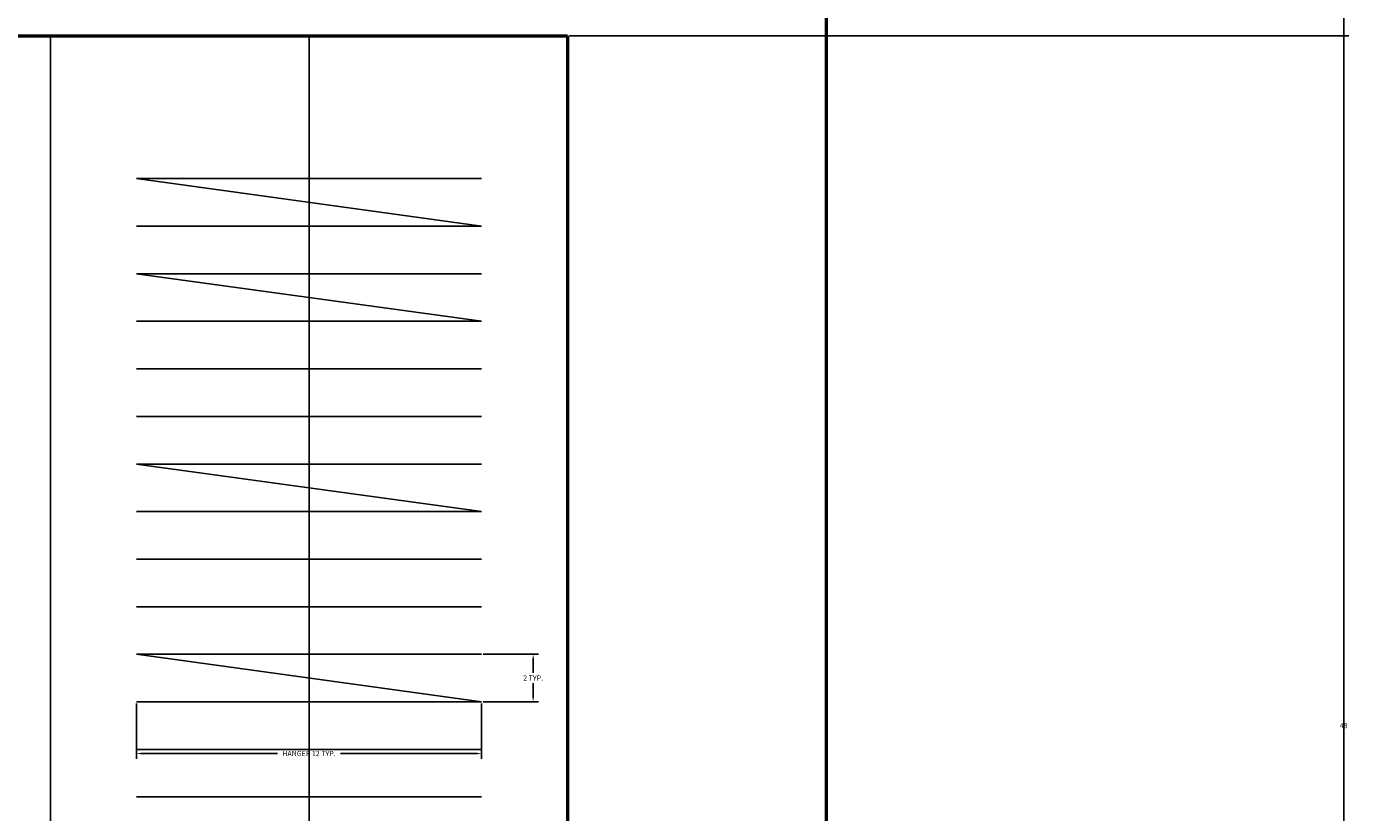
# Model space of a CAD drawing. Units: inches. Extents: x 2621 to 2849, y 2066 to 2463.
# Tile 22 of 28: x 2803 to 2849, y 2344 to 2372. Entities that reach past the tile are written whole.
import ezdxf

# ---------------------------------------------------------------- set-up
doc = ezdxf.new("R2010")
doc.units = ezdxf.units.IN
for name, color, linetype, lineweight in [('A-ANNO-DIMS', 2, 'Continuous', 18), ('A-FLOR-CASE', 9, 'Continuous', 25), ('A-WALL', 7, 'Continuous', 50)]:
    doc.layers.add(name, color=color, linetype=linetype, lineweight=lineweight)
doc.styles.get("Standard").update_dxf_attribs({"font": 'arial.ttf'})
doc.dimstyles.get("Standard").update_dxf_attribs({"dimtxt": 0.18, "dimasz": 0.18, "dimexe": 0.18, "dimexo": 0.0625, "dimgap": 0.09, "dimtad": 0, "dimtih": 1, "dimtoh": 1, "dimdec": 4, "dimzin": 0, "dimdsep": 46, "dimtxsty": 'Standard', "dimcen": 0.09, "dimadec": 0, "dimazin": 0, "dimtfac": 1, "dimtdec": 4, "dimtofl": 0, "dimtmove": 0, "dimatfit": 3, "dimfxl": 1, "dimtolj": 1, "dimtzin": 0, "dimarcsym": 0})

# ---------------------------------------------------------------- blocks, each defined once
blk = doc.blocks.new('CLOSET-HANGER')
for p, q in [((12, 1.655), (0, 1.655)), ((0, 1.655), (12, 0)), ((12, 0), (0, 0))]:
    blk.add_line(p, q)
blk = doc.blocks.new('*D19')
at = {"layer": 'A-ANNO-DIMS', "color": 0, "lineweight": -2, "transparency": 16777216}
for p, q in [((2806.87, 2348.14), (2806.87, 2346.222)), ((2818.87, 2348.14), (2818.87, 2346.222)), ((2807.05, 2346.402), (2811.774, 2346.402)), ((2818.69, 2346.402), (2813.966, 2346.402))]:
    blk.add_line(p, q, dxfattribs=at)
at = {"layer": 'A-ANNO-DIMS', "color": 0, "transparency": 16777216}
for points in [[(2807.05, 2346.432), (2807.05, 2346.372), (2806.87, 2346.402)], [(2818.69, 2346.432), (2818.69, 2346.372), (2818.87, 2346.402)]]:
    blk.add_solid(points, dxfattribs=at)
at = {"layer": 'Defpoints', "color": 0, "transparency": 16777216}
for p in [(2806.87, 2348.202), (2818.87, 2348.202), (2818.87, 2346.402)]:
    blk.add_point(p, dxfattribs=at)
at = {"layer": 'A-ANNO-DIMS', "color": 0, "transparency": 16777216, "insert": (2812.87, 2346.402), "char_height": 0.18, "attachment_point": 5}
blk.add_mtext('\\A1;HANGER 12 TYP.', dxfattribs=at)
blk = doc.blocks.new('*D20')
at = {"layer": 'A-ANNO-DIMS', "color": 0, "lineweight": -2, "transparency": 16777216}
for p, q in [((2818.933, 2349.857), (2820.85, 2349.857)), ((2820.67, 2349.677), (2820.67, 2349.21)), ((2820.67, 2348.382), (2820.67, 2348.849)), ((2818.933, 2348.202), (2820.85, 2348.202))]:
    blk.add_line(p, q, dxfattribs=at)
at = {"layer": 'A-ANNO-DIMS', "color": 0, "transparency": 16777216}
for points in [[(2820.64, 2349.677), (2820.7, 2349.677), (2820.67, 2349.857)], [(2820.64, 2348.382), (2820.7, 2348.382), (2820.67, 2348.202)]]:
    blk.add_solid(points, dxfattribs=at)
at = {"layer": 'Defpoints', "color": 0, "transparency": 16777216}
for p in [(2818.87, 2349.857), (2820.67, 2349.857), (2818.87, 2348.202)]:
    blk.add_point(p, dxfattribs=at)
at = {"layer": 'A-ANNO-DIMS', "color": 0, "transparency": 16777216, "insert": (2820.67, 2349.03), "char_height": 0.18, "attachment_point": 5}
blk.add_mtext('\\A1;2 TYP.', dxfattribs=at)
blk = doc.blocks.new('*D36')
at = {"layer": 'A-ANNO-DIMS', "color": 0, "lineweight": -2, "transparency": 16777216}
for p, q in [((2830.933, 2444.375), (2849.054, 2444.375)), ((2848.874, 2444.195), (2848.874, 2264.557)), ((2848.874, 2084.555), (2848.874, 2264.193)), ((2830.933, 2084.375), (2849.054, 2084.375))]:
    blk.add_line(p, q, dxfattribs=at)
at = {"layer": 'A-ANNO-DIMS', "color": 0, "transparency": 16777216}
for points in [[(2848.844, 2444.195), (2848.904, 2444.195), (2848.874, 2444.375)], [(2848.844, 2084.555), (2848.904, 2084.555), (2848.874, 2084.375)]]:
    blk.add_solid(points, dxfattribs=at)
at = {"layer": 'Defpoints', "color": 0, "transparency": 16777216}
for p in [(2830.87, 2444.375), (2848.874, 2444.375), (2830.87, 2084.375)]:
    blk.add_point(p, dxfattribs=at)
at = {"layer": 'A-ANNO-DIMS', "color": 0, "transparency": 16777216, "insert": (2848.874, 2264.375), "char_height": 0.18, "attachment_point": 5}
blk.add_mtext('\\A1;360', dxfattribs=at)
blk = doc.blocks.new('*D54')
at = {"layer": 'A-ANNO-DIMS', "color": 0, "lineweight": -2, "transparency": 16777216}
for p, q in [((2821.933, 2371.375), (2849.054, 2371.375)), ((2848.874, 2371.195), (2848.874, 2347.556)), ((2848.874, 2323.555), (2848.874, 2347.193)), ((2821.933, 2323.375), (2849.054, 2323.375))]:
    blk.add_line(p, q, dxfattribs=at)
at = {"layer": 'A-ANNO-DIMS', "color": 0, "transparency": 16777216}
for points in [[(2848.844, 2371.195), (2848.904, 2371.195), (2848.874, 2371.375)], [(2848.844, 2323.555), (2848.904, 2323.555), (2848.874, 2323.375)]]:
    blk.add_solid(points, dxfattribs=at)
at = {"layer": 'Defpoints', "color": 0, "transparency": 16777216}
for p in [(2821.87, 2371.375), (2821.87, 2323.375), (2848.874, 2323.375)]:
    blk.add_point(p, dxfattribs=at)
at = {"layer": 'A-ANNO-DIMS', "color": 0, "transparency": 16777216, "insert": (2848.874, 2347.375), "char_height": 0.18, "attachment_point": 5}
blk.add_mtext('\\A1;48', dxfattribs=at)

msp = doc.modelspace()

# ---------------------------------------------------------------- linework, layer by layer
at = {"layer": 'A-FLOR-CASE'}
for p, q in [((2821.8701, 2371.3746), (2803.8701, 2371.3746)), ((2803.8701, 2371.3746), (2803.8701, 2323.3746)), ((2812.8701, 2371.3746), (2812.8701, 2323.3746)), ((2821.8701, 2323.3746), (2821.8701, 2371.3746)), ((2818.8701, 2359.7884), (2806.8701, 2359.7884)), ((2818.8701, 2358.1332), (2806.8701, 2358.1332)), ((2818.8701, 2353.1677), (2806.8701, 2353.1677)), ((2818.8701, 2351.5125), (2806.8701, 2351.5125)), ((2818.8701, 2346.547), (2806.8701, 2346.547)), ((2818.8701, 2344.8918), (2806.8701, 2344.8918))]:
    msp.add_line(p, q, dxfattribs=at)
at = {"layer": 'A-WALL'}
for p, q in [((2797.8701, 2371.3746), (2821.8701, 2371.3746)), ((2821.8701, 2371.3746), (2821.8701, 2319.3746)), ((2821.8701, 2371.3746), (2821.8701, 2093.3746))]:
    msp.add_line(p, q, dxfattribs=at)
msp.add_lwpolyline([(2761.8701, 2084.3746), (2638.8701, 2084.3746), (2638.8701, 2444.3746), (2830.8701, 2444.3746), (2830.8701, 2084.3746), (2797.8701, 2084.3746)], dxfattribs=at)

# ---------------------------------------------------------------- block references
at = {"layer": 'A-FLOR-CASE'}
for p in [(2806.87, 2364.754), (2806.87, 2361.4437), (2806.87, 2354.823), (2806.87, 2348.2023)]:
    msp.add_blockref('CLOSET-HANGER', p, dxfattribs=at)

# ---------------------------------------------------------------- dimensions: what is measured, and where the dimension line sits
at = {"layer": 'A-ANNO-DIMS'}
for base, p1, p2, picture, middle in [((2848.8736, 2444.3746), (2830.8701, 2084.3746), (2830.8701, 2444.3746), '*D36', (2848.8736, 2264.3746)), ((2848.8736, 2323.3746), (2821.8701, 2371.3746), (2821.8701, 2323.3746), '*D54', (2848.8736, 2347.3746))]:
    dim = msp.add_linear_dim(base=base, p1=p1, p2=p2, angle=90, dimstyle='Standard', override={"dimdec": 0, "dimlfac": 1, "dimrnd": 0, "dimzin": 0, "dimdsep": 46, "dimlunit": 2}, dxfattribs=at)
    dim.commit()
    dim.dimension.update_dxf_attribs({"geometry": picture, "text_midpoint": middle})
dim = msp.add_linear_dim(base=(2820.6701, 2349.8573), p1=(2818.8701, 2348.2022), p2=(2818.8701, 2349.8573), angle=90, text='<> TYP.', dimstyle='Standard', override={"dimdec": 0, "dimlfac": 1, "dimrnd": 0, "dimzin": 0, "dimdsep": 46, "dimlunit": 2}, dxfattribs=at)
dim.commit()
dim.dimension.update_dxf_attribs({"geometry": '*D20', "text_midpoint": (2820.6701, 2349.0298)})
dim = msp.add_linear_dim(base=(2818.8701, 2346.4022), p1=(2806.8701, 2348.2022), p2=(2818.8701, 2348.2022), text='HANGER <> TYP.', dimstyle='Standard', override={"dimdec": 0, "dimlfac": 1, "dimrnd": 0, "dimzin": 0, "dimdsep": 46, "dimlunit": 2}, dxfattribs=at)
dim.commit()
dim.dimension.update_dxf_attribs({"geometry": '*D19', "text_midpoint": (2812.8701, 2346.4022)})

doc.saveas('drawing.dxf')
